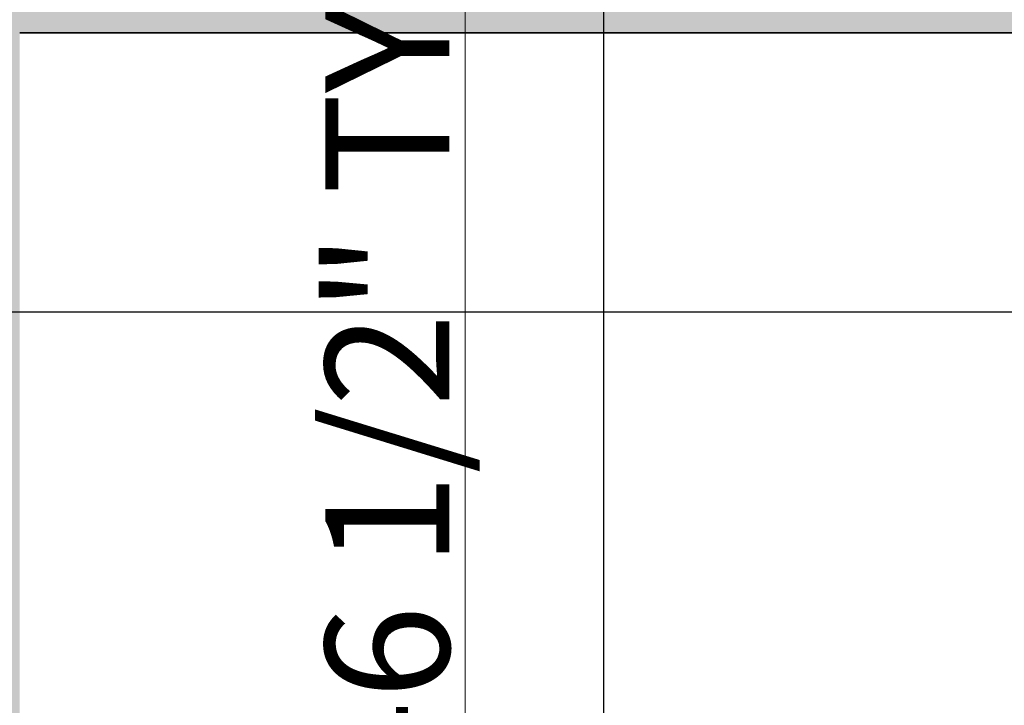
# Model space of a CAD drawing. Units: inches. Extents: x 2696 to 3240, y 1564 to 2310.
# Tile 49 of 76: x 2755 to 2802, y 2104 to 2137. Entities that reach past the tile are written whole.
import ezdxf

# ---------------------------------------------------------------- set-up
doc = ezdxf.new("R2010")
doc.units = ezdxf.units.IN
for name, color, linetype, lineweight in [('A-ANNO-DIMS', 3, 'Continuous', 18), ('A-WALL', 7, 'Continuous', 35), ('A-WALL-PATT', 9, 'Continuous', 13)]:
    doc.layers.add(name, color=color, linetype=linetype, lineweight=lineweight)
doc.styles.add('TIMES NEW', font='times.ttf')
doc.dimstyles.new('Siddhuu', dxfattribs={"dimtxt": 6, "dimasz": 2.5, "dimexe": 1.25, "dimexo": 0.625, "dimtad": 1, "dimdec": 1, "dimlunit": 4, "dimtxsty": 'TIMES NEW', "dimcen": 2.5, "dimclrd": 256, "dimclre": 1, "dimclrt": 7, "dimadec": 0, "dimazin": 0, "dimtfac": 1, "dimtdec": 1, "dimtmove": 0, "dimatfit": 3, "dimfxl": 1, "dimtolj": 1, "dimlwd": -1, "dimarcsym": 0})

# ---------------------------------------------------------------- blocks, each defined once
blk = doc.blocks.new('*D40')
at = {"layer": 'A-ANNO-DIMS', "color": 1, "lineweight": -2, "transparency": 16777216}
for p, q in [((2777.266, 2091.826), (2777.266, 2093.576)), ((2784.764, 2091.826), (2784.764, 2093.576))]:
    blk.add_line(p, q, dxfattribs=at)
at = {"layer": 'A-ANNO-DIMS', "transparency": 16777216}
for p, q in [((2779.766, 2092.326), (2782.264, 2092.326)), ((2784.764, 2092.326), (2902.458, 2092.326))]:
    blk.add_line(p, q, dxfattribs=at)
for points in [[(2779.766, 2092.742), (2779.766, 2091.909), (2777.266, 2092.326)], [(2782.264, 2092.742), (2782.264, 2091.909), (2784.764, 2092.326)]]:
    blk.add_solid(points, dxfattribs=at)
at = {"layer": 'Defpoints', "color": 0, "transparency": 16777216}
for p in [(2784.764, 2092.326), (2777.266, 2091.201), (2784.764, 2091.201)]:
    blk.add_point(p, dxfattribs=at)
at = {"layer": 'A-ANNO-DIMS', "color": 7, "transparency": 16777216, "insert": (2844.861, 2096.094), "char_height": 6, "attachment_point": 5, "style": 'TIMES NEW'}
blk.add_mtext('\\A1;BATH FITTING 0\'-7 1/2" TYP.', dxfattribs=at)
blk = doc.blocks.new('*D41')
at = {"layer": 'A-ANNO-DIMS', "transparency": 16777216}
for p, q in [((2776.142, 2091.201), (2776.142, 2145.728)), ((2776.142, 2087.2), (2776.142, 2088.701))]:
    blk.add_line(p, q, dxfattribs=at)
at = {"layer": 'A-ANNO-DIMS', "color": 1, "lineweight": -2, "transparency": 16777216}
for p, q in [((2776.641, 2091.201), (2774.892, 2091.201)), ((2776.641, 2084.7), (2774.892, 2084.7))]:
    blk.add_line(p, q, dxfattribs=at)
at = {"layer": 'A-ANNO-DIMS', "transparency": 16777216}
for points in [[(2775.725, 2088.701), (2776.558, 2088.701), (2776.142, 2091.201)], [(2775.725, 2087.2), (2776.558, 2087.2), (2776.142, 2084.7)]]:
    blk.add_solid(points, dxfattribs=at)
at = {"layer": 'Defpoints', "color": 0, "transparency": 16777216}
for p in [(2776.142, 2091.201), (2777.266, 2091.201), (2777.266, 2084.7)]:
    blk.add_point(p, dxfattribs=at)
at = {"layer": 'A-ANNO-DIMS', "color": 7, "transparency": 16777216, "insert": (2772.38, 2119.715), "char_height": 6, "attachment_point": 5, "rotation": 90, "style": 'TIMES NEW'}
blk.add_mtext('\\A1;0\'-6 1/2" TYP.', dxfattribs=at)
blk = doc.blocks.new('*D62')
at = {"layer": 'A-ANNO-DIMS', "color": 1, "lineweight": -2, "transparency": 16777216}
for p, q in [((2965.084, 2140.701), (2709.361, 2140.701)), ((2965.084, 2063.591), (2709.361, 2063.591))]:
    blk.add_line(p, q, dxfattribs=at)
at = {"layer": 'A-ANNO-DIMS', "transparency": 16777216}
blk.add_line((2710.611, 2066.091), (2710.611, 2138.201), dxfattribs=at)
for points in [[(2710.195, 2138.201), (2711.028, 2138.201), (2710.611, 2140.701)], [(2710.195, 2066.091), (2711.028, 2066.091), (2710.611, 2063.591)]]:
    blk.add_solid(points, dxfattribs=at)
at = {"layer": 'Defpoints', "color": 0, "transparency": 16777216}
for p in [(2710.611, 2140.701), (2965.709, 2140.701), (2965.709, 2063.591)]:
    blk.add_point(p, dxfattribs=at)
at = {"layer": 'A-ANNO-DIMS', "color": 7, "transparency": 16777216, "insert": (2706.934, 2102.146), "char_height": 6, "attachment_point": 5, "rotation": 90, "style": 'TIMES NEW'}
blk.add_mtext('\\A1;6\'-5"', dxfattribs=at)
blk = doc.blocks.new('*D64')
at = {"layer": 'A-ANNO-DIMS', "color": 1, "lineweight": -2, "transparency": 16777216}
for p, q in [((3073.084, 2206.701), (2709.361, 2206.701)), ((3068.584, 1989.201), (2709.361, 1989.201))]:
    blk.add_line(p, q, dxfattribs=at)
at = {"layer": 'A-ANNO-DIMS', "transparency": 16777216}
blk.add_line((2710.611, 1991.701), (2710.611, 2204.201), dxfattribs=at)
for points in [[(2710.195, 2204.201), (2711.028, 2204.201), (2710.611, 2206.701)], [(2710.195, 1991.701), (2711.028, 1991.701), (2710.611, 1989.201)]]:
    blk.add_solid(points, dxfattribs=at)
at = {"layer": 'Defpoints', "color": 0, "transparency": 16777216}
for p in [(2710.611, 2206.701), (3073.709, 2206.701), (3069.209, 1989.201)]:
    blk.add_point(p, dxfattribs=at)
at = {"layer": 'A-ANNO-DIMS', "color": 7, "transparency": 16777216, "insert": (2706.85, 2097.951), "char_height": 6, "attachment_point": 5, "rotation": 90, "style": 'TIMES NEW'}
blk.add_mtext('\\A1;18\'-1 1/2"', dxfattribs=at)
blk = doc.blocks.new('*D66')
at = {"layer": 'A-ANNO-DIMS', "color": 1, "lineweight": -2, "transparency": 16777216}
for p, q in [((3077.584, 2122.701), (2709.361, 2122.701)), ((3077.584, 2074.701), (2709.361, 2074.701))]:
    blk.add_line(p, q, dxfattribs=at)
at = {"layer": 'A-ANNO-DIMS', "transparency": 16777216}
blk.add_line((2710.611, 2077.201), (2710.611, 2120.201), dxfattribs=at)
for points in [[(2710.195, 2120.201), (2711.028, 2120.201), (2710.611, 2122.701)], [(2710.195, 2077.201), (2711.028, 2077.201), (2710.611, 2074.701)]]:
    blk.add_solid(points, dxfattribs=at)
at = {"layer": 'Defpoints', "color": 0, "transparency": 16777216}
for p in [(2710.611, 2122.701), (3078.209, 2122.701), (3078.209, 2074.701)]:
    blk.add_point(p, dxfattribs=at)
at = {"layer": 'A-ANNO-DIMS', "color": 7, "transparency": 16777216, "insert": (2706.934, 2098.701), "char_height": 6, "attachment_point": 5, "rotation": 90, "style": 'TIMES NEW'}
blk.add_mtext('\\A1;4\'-0"', dxfattribs=at)
blk = doc.blocks.new('*D68')
at = {"layer": 'A-ANNO-DIMS', "color": 1, "lineweight": -2, "transparency": 16777216}
for p, q in [((2745.611, 2261.576), (2745.611, 1568.951)), ((2782.834, 2261.576), (2782.834, 1568.951))]:
    blk.add_line(p, q, dxfattribs=at)
at = {"layer": 'A-ANNO-DIMS', "transparency": 16777216}
blk.add_line((2748.111, 1570.201), (2780.334, 1570.201), dxfattribs=at)
for points in [[(2748.111, 1570.618), (2748.111, 1569.784), (2745.611, 1570.201)], [(2780.334, 1570.618), (2780.334, 1569.784), (2782.834, 1570.201)]]:
    blk.add_solid(points, dxfattribs=at)
at = {"layer": 'Defpoints', "color": 0, "transparency": 16777216}
for p in [(2745.611, 2262.201), (2782.834, 2262.201), (2782.834, 1570.201)]:
    blk.add_point(p, dxfattribs=at)
at = {"layer": 'A-ANNO-DIMS', "color": 7, "transparency": 16777216, "insert": (2764.223, 1573.878), "char_height": 6, "attachment_point": 5, "style": 'TIMES NEW'}
blk.add_mtext('\\A1;3\'-1"', dxfattribs=at)

msp = doc.modelspace()

# ---------------------------------------------------------------- hatches: boundary and pattern name
at = {"layer": 'A-WALL-PATT', "transparency": 33554556}
h = msp.add_hatch(color=256, dxfattribs=at)
h.dxf.hatch_style = 1
h.paths.add_polyline_path([(2879.111, 2253.201), (2905.91, 2253.201), (2905.91, 2262.201), (2841.889, 2262.201), (2841.889, 2253.201), (2870.111, 2253.201), (2870.111, 2176.601), (2965.709, 2176.601), (2965.709, 2206.701), (2973.583, 2206.701), (2973.583, 2215.701), (2965.709, 2215.701), (2965.709, 2262.201), (2929.91, 2262.201), (2929.91, 2253.201), (2956.709, 2253.201), (2956.709, 2185.601), (2879.111, 2185.601)])
h.paths.add_polyline_path([(2782.834, 2262.201), (2745.611, 2262.201), (2745.611, 2228.729), (2754.611, 2228.729), (2754.611, 2253.201), (2782.834, 2253.201)])
h.paths.add_polyline_path([(2754.611, 2136.201), (2965.709, 2136.201), (2965.709, 2145.201), (2879.111, 2145.201), (2879.111, 2147.074), (2877.34, 2147.074), (2870.111, 2147.074), (2870.111, 2145.201), (2754.611, 2145.201), (2754.611, 2169.674), (2745.611, 2169.674), (2745.611, 2000.201), (2754.611, 2000.201), (2754.611, 2019.201), (2849.083, 2019.201), (2849.083, 2023.701), (2841.209, 2023.701), (2841.209, 2051.827), (2836.709, 2051.827), (2836.709, 2023.701), (2754.611, 2023.701), (2754.611, 2091.201), (2836.709, 2091.201), (2836.709, 2087.827), (2841.209, 2087.827), (2841.209, 2095.701), (2754.611, 2095.701)])
h.paths.add_polyline_path([(2965.709, 2136.201), (2956.709, 2136.201), (2956.709, 2023.701), (2885.083, 2023.701), (2885.083, 2019.201), (2956.709, 2019.201), (2956.709, 1950.575), (2965.709, 1950.575), (2965.709, 1980.201), (2973.583, 1980.201), (2973.583, 1989.201), (2965.709, 1989.201)])
h.paths.add_polyline_path([(2754.611, 1906.701), (2880.209, 1906.701), (2884.709, 1906.701), (2956.709, 1906.701), (2956.709, 1792.701), (2944.709, 1792.701), (2944.709, 1783.701), (2956.709, 1783.701), (2956.709, 1740.201), (2884.709, 1740.201), (2884.709, 1783.701), (2896.709, 1783.701), (2896.709, 1792.701), (2884.709, 1792.701), (2884.709, 1846.701), (2880.209, 1846.701), (2880.209, 1740.201), (2754.611, 1740.201), (2754.611, 1777.201), (2745.611, 1777.201), (2745.611, 1692.701), (2754.611, 1692.701), (2754.611, 1731.201), (2956.709, 1731.201), (2956.709, 1723.327), (2965.709, 1723.327), (2965.709, 1884.201), (2973.583, 1884.201), (2973.583, 1893.201), (2965.709, 1893.201), (2965.709, 1914.575), (2956.709, 1914.575), (2956.709, 1911.201), (2754.611, 1911.201), (2754.611, 1930.201), (2745.611, 1930.201), (2745.611, 1817.201), (2754.611, 1817.201), (2754.611, 1854.201), (2826.611, 1854.201), (2826.611, 1868.827), (2822.111, 1868.827), (2822.111, 1858.701), (2754.611, 1858.701)])
h.paths.add_polyline_path([(2965.709, 1656.201), (3008.237, 1656.201), (3008.237, 1665.201), (2965.709, 1665.201), (2965.709, 1693.327), (2956.709, 1693.327), (2956.709, 1686.201), (2934.583, 1686.201), (2934.583, 1681.701), (2956.709, 1681.701), (2956.709, 1614.201), (2896.709, 1614.201), (2896.709, 1681.701), (2904.583, 1681.701), (2904.583, 1686.201), (2892.209, 1686.201), (2892.209, 1614.201), (2858.41, 1614.201), (2858.41, 1605.201), (2965.709, 1605.201)])
h.paths.add_polyline_path([(2788.41, 1614.201), (2754.611, 1614.201), (2754.611, 1652.701), (2745.611, 1652.701), (2745.611, 1605.201), (2788.41, 1605.201)])
h.paths.add_polyline_path([(3199.611, 1633.048), (3190.611, 1633.048), (3190.611, 1614.201), (3082.611, 1614.201), (3082.611, 1665.201), (3070.237, 1665.201), (3070.237, 1656.201), (3078.111, 1656.201), (3078.111, 1605.201), (3199.611, 1605.201)])
h.paths.add_polyline_path([(3199.611, 1702.048), (3190.611, 1702.048), (3190.611, 1699.701), (3106.611, 1699.701), (3106.611, 1747.701), (3190.611, 1747.701), (3190.611, 1752.201), (3082.611, 1752.201), (3082.611, 1760.075), (3078.111, 1760.075), (3078.111, 1747.701), (3102.111, 1747.701), (3102.111, 1699.701), (3078.111, 1699.701), (3078.111, 1695.201), (3190.611, 1695.201), (3190.611, 1676.355), (3199.611, 1676.355)])
h.paths.add_polyline_path([(3199.611, 1783.201), (3190.611, 1783.201), (3190.611, 1745.355), (3199.611, 1745.355)])
h.paths.add_polyline_path([(3082.611, 1884.201), (3190.611, 1884.201), (3190.611, 1853.201), (3199.611, 1853.201), (3199.611, 1901.701), (3190.611, 1901.701), (3190.611, 1893.201), (3005.583, 1893.201), (3005.583, 1891.281), (3005.583, 1884.201), (3078.111, 1884.201), (3078.111, 1792.075), (3082.611, 1792.075)])
h.paths.add_polyline_path([(3199.611, 1994.701), (3190.611, 1994.701), (3190.611, 1989.201), (3073.709, 1989.201), (3073.709, 2034.201), (3069.209, 2034.201), (3069.209, 1989.201), (3005.583, 1989.201), (3005.583, 1980.201), (3190.611, 1980.201), (3190.611, 1971.701), (3199.611, 1971.701)])
h.paths.add_polyline_path([(3199.611, 2155.201), (3190.611, 2155.201), (3190.611, 2064.701), (3199.611, 2064.701)])
h.paths.add_polyline_path([(3190.611, 2074.701), (3106.611, 2074.701), (3106.611, 2122.701), (3190.611, 2122.701), (3190.611, 2127.201), (3082.709, 2127.201), (3082.709, 2135.075), (3073.709, 2135.075), (3073.709, 2122.701), (3102.111, 2122.701), (3102.111, 2074.701), (3069.209, 2074.701), (3069.209, 2070.201), (3190.611, 2070.201)])
h.paths.add_polyline_path([(3082.709, 2253.201), (3190.611, 2253.201), (3190.611, 2225.201), (3199.611, 2225.201), (3199.611, 2262.201), (3073.709, 2262.201), (3073.709, 2215.701), (3035.583, 2215.701), (3035.583, 2206.701), (3073.709, 2206.701), (3073.709, 2171.075), (3082.709, 2171.075)])

# ---------------------------------------------------------------- linework, layer by layer
at = {"layer": 'A-WALL'}
msp.add_line((2754.611, 2136.201), (2965.709, 2136.201), dxfattribs=at)

# ---------------------------------------------------------------- dimensions: what is measured, and where the dimension line sits
at = {"layer": 'A-ANNO-DIMS'}
dim = msp.add_linear_dim(base=(2782.834, 1570.201), p1=(2745.611, 2262.201), p2=(2782.834, 2262.201), dimstyle='Siddhuu', override={"dimdec": 1, "dimlfac": 1, "dimrnd": 0, "dimzin": 1, "dimdsep": 46, "dimlunit": 4, "dimfrac": 2}, dxfattribs=at)
dim.commit()
dim.dimension.update_dxf_attribs({"geometry": '*D68', "text_midpoint": (2764.223, 1573.878)})
for base, p1, p2, picture, middle in [((2710.611, 2206.701), (3069.209, 1989.201), (3073.709, 2206.701), '*D64', (2706.85, 2097.951)), ((2710.611, 2140.701), (2965.709, 2063.591), (2965.709, 2140.701), '*D62', (2706.934, 2102.146)), ((2710.611, 2122.701), (3078.209, 2074.701), (3078.209, 2122.701), '*D66', (2706.934, 2098.701))]:
    dim = msp.add_linear_dim(base=base, p1=p1, p2=p2, angle=90, dimstyle='Siddhuu', override={"dimdec": 1, "dimlfac": 1, "dimrnd": 0, "dimzin": 1, "dimdsep": 46, "dimlunit": 4, "dimfrac": 2}, dxfattribs=at)
    dim.commit()
    dim.dimension.update_dxf_attribs({"geometry": picture, "text_midpoint": middle})
dim = msp.add_linear_dim(base=(2776.142, 2091.201), p1=(2777.266, 2084.7), p2=(2777.266, 2091.201), angle=90, text='<> TYP.', dimstyle='Siddhuu', override={"dimdec": 1, "dimlfac": 1, "dimrnd": 0, "dimzin": 1, "dimdsep": 46, "dimlunit": 4, "dimfrac": 2}, dxfattribs=at)
dim.commit()
dim.dimension.update_dxf_attribs({"geometry": '*D41', "text_midpoint": (2772.38, 2119.715)})
dim = msp.add_linear_dim(base=(2784.764, 2092.326), p1=(2777.266, 2091.201), p2=(2784.764, 2091.201), text='BATH FITTING <> TYP.', dimstyle='Siddhuu', override={"dimdec": 1, "dimlfac": 1, "dimrnd": 0, "dimzin": 1, "dimdsep": 46, "dimlunit": 4, "dimfrac": 2}, dxfattribs=at)
dim.commit()
dim.dimension.update_dxf_attribs({"geometry": '*D40', "text_midpoint": (2844.861, 2096.094)})

doc.saveas('drawing.dxf')
